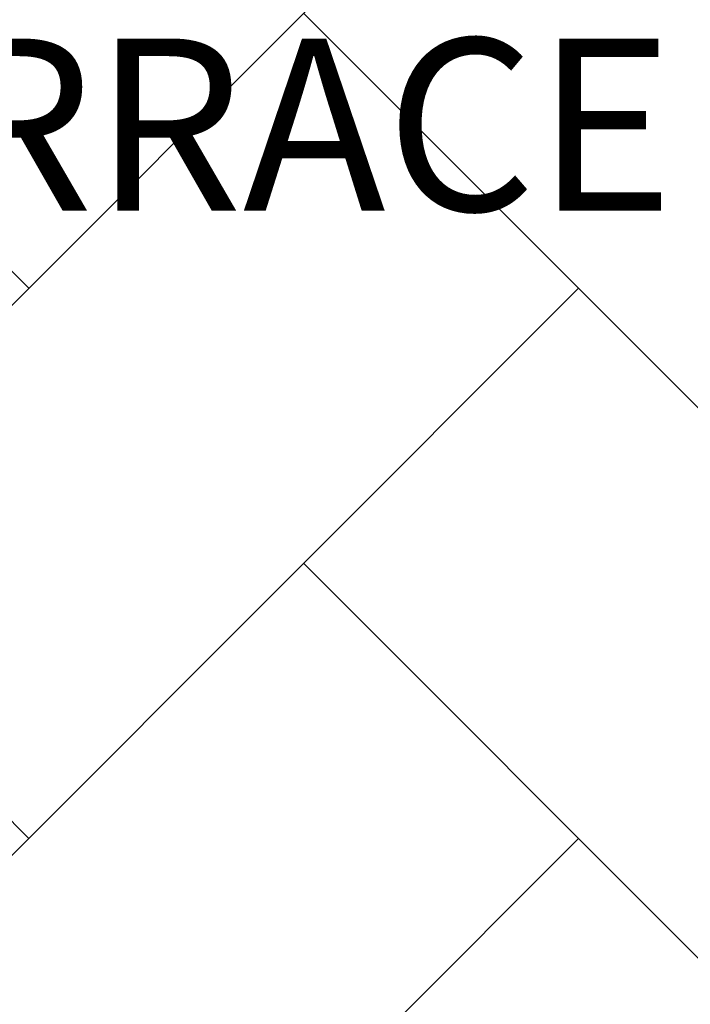
# Model space of a CAD drawing. Units: inches. Extents: x 3590 to 5167, y 65 to 1917.
# Tile 59 of 100: x 5000 to 5035, y 1558 to 1609. Entities that reach past the tile are written whole.
import ezdxf

# ---------------------------------------------------------------- set-up
doc = ezdxf.new("R2010")
doc.units = ezdxf.units.IN
doc.layers.add('A-AREA-IDEN', color=7, linetype='Continuous', lineweight=18)
doc.layers.add('A-FLOR-PATT', color=8, linetype='Continuous', lineweight=13)
doc.styles.get("Standard").update_dxf_attribs({"font": 'arial.ttf'})

msp = doc.modelspace()

# ---------------------------------------------------------------- hatches: boundary and pattern name
at = {"layer": 'A-FLOR-PATT', "transparency": 33554687}
h = msp.add_hatch(dxfattribs=at)
h.set_pattern_fill('AR-HBONE', color=256, scale=0.2)
h.set_pattern_definition([(45, (-588.972, 0), (0, 28.73682), [60.96, -20.32]), (135, (-574.604, 14.368), (3e-15, 28.73682), [60.96, -20.32])])
h.paths.add_polyline_path([(5071.274, 1796.999), (4933.274, 1796.999), (4933.274, 1753.999), (4962.774, 1753.999, -0.414214), (4928.774, 1719.999), (4933.274, 1718.999), (4933.274, 1334.999), (5071.274, 1334.999)])
h.paths.add_polyline_path([(4951.78, 1521.077), (4951.715, 1521.04), (4951.563, 1520.895)], flags=16)
h.paths.add_polyline_path([(4952.267, 1521.376), (4952.198, 1521.371), (4952.198, 1521.356)], flags=0)
h.paths.add_polyline_path([(4967.051, 1529.728), (4965.231, 1528.694), (4963.411, 1527.714), (4961.756, 1526.851), (4963.589, 1527.449), (4964.036, 1527.478), (4962.975, 1527.249), (4961.76, 1526.852), (4959.792, 1525.834), (4958.005, 1524.895), (4956.24, 1523.93), (4954.504, 1522.919), (4954.129, 1522.682), (4953.361, 1521.997), (4953.366, 1521.998), (4953.605, 1522.064), (4955.106, 1522.761), (4956.921, 1523.434), (4958.678, 1523.915), (4960.358, 1524.2), (4961.945, 1524.286), (4964.171, 1524.108), (4965.958, 1523.309), (4963.863, 1522.976), (4965.187, 1522.499), (4963.366, 1522.497), (4961.545, 1522.487), (4959.764, 1522.461), (4958.304, 1522.419), (4957.974, 1522.388), (4956.307, 1522.232), (4954.718, 1522.071), (4953.251, 1521.899), (4953.525, 1521.623), (4954.331, 1521.379), (4956.243, 1521.23), (4958.039, 1520.93), (4959.684, 1520.483), (4961.16, 1519.896), (4963.107, 1518.8), (4964.393, 1517.325), (4962.973, 1517.726), (4964.558, 1516.661), (4965.407, 1515.708), (4963.507, 1516.322), (4961.68, 1517.005), (4959.935, 1517.745), (4958.282, 1518.528), (4956.732, 1519.343), (4955.295, 1520.175), (4954.672, 1520.572), (4954.513, 1520.627), (4955.658, 1519.318), (4956.703, 1517.982), (4957.644, 1516.647), (4958.485, 1515.334), (4959.55, 1513.524), (4960.438, 1511.769), (4958.841, 1513.62), (4957.452, 1515.325), (4955.819, 1517.459), (4956.665, 1515.448), (4957.111, 1513.923), (4957.447, 1511.714), (4957.076, 1509.793), (4956.538, 1511.11), (4955.992, 1512.569), (4955.444, 1514.125), (4954.898, 1515.735), (4954.357, 1517.356), (4953.824, 1518.943), (4953.305, 1520.452), (4953.065, 1521.116), (4952.971, 1521.146), (4952.949, 1521.086), (4952.73, 1520.199), (4953.37, 1518.024), (4953.757, 1516.373), (4954.051, 1514.765), (4954.264, 1513.221), (4954.471, 1511.131), (4954.497, 1510.402), (4954.409, 1511.76), (4954.264, 1513.221), (4954.051, 1514.765), (4953.757, 1516.373), (4953.37, 1518.024), (4952.877, 1519.698), (4952.716, 1520.141), (4952.533, 1519.059), (4952.374, 1517.789), (4952.219, 1516.312), (4952.046, 1514.6), (4951.833, 1512.626), (4951.557, 1510.363), (4951.203, 1512.168), (4950.852, 1514.339), (4950.985, 1516.376), (4951.66, 1518.286), (4952.593, 1520.481), (4952.357, 1521.13), (4951.855, 1520.328), (4950.839, 1518.908), (4949.777, 1517.587), (4948.916, 1516.617), (4948.111, 1515.256), (4947.089, 1513.554), (4945.889, 1511.615), (4946.326, 1513.402), (4946.562, 1514.249), (4945.528, 1513.327), (4944.581, 1512.531), (4946.018, 1514.508), (4947.204, 1516.048), (4947.893, 1517.313), (4949.307, 1518.764), (4950.414, 1519.767), (4950.451, 1519.806), (4952.267, 1521.376), (4951.645, 1521.493), (4950.404, 1521.18), (4948.044, 1520.359), (4946.119, 1519.452), (4944.572, 1518.475), (4943.35, 1517.443), (4941.997, 1515.92), (4941.661, 1515.275), (4942.813, 1516.99), (4944.572, 1518.475), (4946.119, 1519.452), (4948.044, 1520.359), (4950.404, 1521.18), (4951.645, 1521.493), (4949.647, 1521.868), (4948.6, 1521.756), (4947.126, 1521.57), (4945.42, 1521.348), (4943.45, 1521.105), (4941.183, 1520.856), (4942.86, 1521.613), (4943.873, 1522.03), (4942.952, 1521.909), (4941.41, 1521.485), (4939.543, 1520.67), (4938.968, 1520.226), (4940.733, 1521.299), (4942.952, 1521.909), (4943.702, 1522.008), (4945.894, 1522.7), (4947.565, 1522.714), (4948.921, 1522.566), (4951.131, 1522.183), (4950.971, 1522.297), (4948.129, 1523.006), (4946.035, 1523.707), (4944.232, 1524.521), (4942.707, 1525.461), (4941.444, 1526.537), (4940.43, 1527.761), (4939.649, 1529.143), (4941.421, 1528.122), (4943.147, 1527.132), (4944.841, 1526.175), (4946.514, 1525.25), (4948.179, 1524.359), (4948.365, 1524.263), (4946.475, 1526.045), (4945.181, 1527.54), (4944.19, 1529.033), (4943.496, 1530.54), (4943.278, 1531.36), (4942.498, 1531.919), (4943.114, 1531.762), (4942.959, 1533.659), (4944.14, 1531.989), (4944.612, 1531.323), (4946.202, 1530.463), (4947.486, 1529.509), (4948.79, 1528.226), (4950.368, 1526.237), (4949.485, 1528.155), (4948.851, 1530.123), (4948.491, 1532.041), (4948.381, 1533.918), (4948.501, 1535.76), (4948.827, 1537.573), (4949.418, 1535.565), (4949.957, 1533.569), (4950.464, 1531.586), (4950.961, 1529.617), (4951.391, 1527.954), (4951.724, 1530.687), (4952.201, 1532.58), (4952.889, 1534.33), (4953.77, 1535.951), (4954.827, 1537.46), (4954.521, 1535.39), (4954.273, 1533.937), (4955.58, 1535.663), (4956.748, 1536.739), (4956.159, 1534.78), (4955.589, 1532.873), (4955.043, 1531.006), (4954.525, 1529.166), (4954.038, 1527.341), (4953.638, 1525.733), (4953.611, 1525.586), (4953.398, 1524.166), (4953.382, 1524.009), (4954.07, 1525.476), (4954.912, 1527.022), (4956.136, 1528.894), (4957.847, 1530.577), (4959.376, 1531.54), (4958.256, 1530.104), (4957.143, 1528.663), (4956.066, 1527.243), (4955.056, 1525.871), (4954.141, 1524.571), (4953.352, 1523.372), (4953.311, 1523.303), (4953.273, 1522.925), (4953.261, 1522.382), (4954.103, 1523.373), (4954.63, 1524.284), (4955.961, 1526.358), (4957.23, 1528.13), (4958.421, 1529.609), (4960.037, 1531.368), (4961.374, 1532.375), (4962.101, 1532.77), (4961.07, 1531.061), (4959.987, 1529.438), (4958.869, 1527.908), (4958.15, 1527.007), (4959.803, 1528.003), (4961.589, 1528.793), (4963.391, 1529.328), (4965.211, 1529.632)], flags=16)
h.paths.add_polyline_path([(4962.944, 1523.182), (4961.107, 1523.422), (4960.392, 1523.362), (4962.35, 1523.331)], flags=0)
h.paths.add_polyline_path([(5049.541, 1584.551), (5049.476, 1584.515), (5049.325, 1584.37)], flags=16)
h.paths.add_polyline_path([(5050.028, 1584.851), (5049.959, 1584.845), (5049.959, 1584.83)], flags=0)
h.paths.add_polyline_path([(5042.333, 1581.949), (5043.88, 1582.926), (5045.806, 1583.833), (5048.165, 1584.654), (5049.406, 1584.967), (5047.408, 1585.342), (5046.361, 1585.231), (5044.888, 1585.044), (5043.181, 1584.822), (5041.211, 1584.579), (5038.944, 1584.33), (5040.622, 1585.087), (5041.634, 1585.504), (5040.713, 1585.383), (5039.171, 1584.959), (5037.304, 1584.144), (5036.729, 1583.7), (5038.494, 1584.773), (5040.713, 1585.383), (5041.463, 1585.482), (5043.655, 1586.174), (5045.326, 1586.188), (5046.682, 1586.04), (5048.893, 1585.657), (5048.732, 1585.771), (5045.891, 1586.48), (5043.796, 1587.181), (5041.994, 1587.996), (5040.468, 1588.935), (5039.205, 1590.011), (5038.191, 1591.235), (5037.41, 1592.617), (5039.182, 1591.596), (5040.909, 1590.607), (5042.602, 1589.649), (5044.275, 1588.724), (5045.94, 1587.833), (5046.126, 1587.738), (5044.237, 1589.519), (5042.942, 1591.015), (5041.952, 1592.508), (5041.257, 1594.014), (5041.039, 1594.834), (5040.26, 1595.393), (5040.875, 1595.237), (5040.721, 1597.133), (5041.901, 1595.463), (5042.373, 1594.798), (5043.963, 1593.938), (5045.247, 1592.983), (5046.552, 1591.701), (5048.129, 1589.712), (5047.247, 1591.63), (5046.613, 1593.597), (5046.252, 1595.515), (5046.142, 1597.392), (5046.262, 1599.234), (5046.588, 1601.047), (5047.179, 1599.039), (5047.718, 1597.043), (5048.225, 1595.06), (5048.722, 1593.091), (5049.152, 1591.429), (5049.485, 1594.161), (5049.962, 1596.054), (5050.65, 1597.804), (5051.532, 1599.425), (5052.589, 1600.934), (5052.283, 1598.864), (5052.034, 1597.411), (5053.341, 1599.137), (5054.509, 1600.213), (5053.92, 1598.254), (5053.35, 1596.348), (5052.805, 1594.48), (5052.286, 1592.64), (5051.799, 1590.815), (5051.4, 1589.207), (5051.373, 1589.06), (5051.159, 1587.64), (5051.143, 1587.483), (5051.831, 1588.95), (5052.673, 1590.496), (5053.898, 1592.368), (5055.608, 1594.051), (5057.137, 1595.014), (5056.017, 1593.578), (5054.904, 1592.137), (5053.828, 1590.717), (5052.817, 1589.345), (5051.902, 1588.046), (5051.113, 1586.846), (5051.072, 1586.777), (5051.034, 1586.399), (5051.022, 1585.856), (5051.864, 1586.847), (5052.391, 1587.758), (5053.723, 1589.832), (5054.991, 1591.604), (5056.182, 1593.083), (5057.798, 1594.842), (5059.135, 1595.849), (5059.863, 1596.244), (5058.831, 1594.535), (5057.749, 1592.912), (5056.63, 1591.382), (5055.912, 1590.482), (5057.564, 1591.477), (5059.35, 1592.267), (5061.152, 1592.802), (5062.972, 1593.106), (5064.812, 1593.203), (5062.992, 1592.169), (5061.172, 1591.188), (5059.518, 1590.325), (5061.35, 1590.924), (5061.797, 1590.952), (5060.737, 1590.723), (5059.521, 1590.326), (5057.553, 1589.308), (5055.766, 1588.369), (5054.002, 1587.404), (5052.265, 1586.393), (5051.891, 1586.156), (5051.122, 1585.471), (5051.127, 1585.472), (5051.366, 1585.538), (5052.867, 1586.235), (5054.682, 1586.908), (5056.439, 1587.389), (5058.12, 1587.675), (5059.706, 1587.76), (5061.933, 1587.583), (5063.719, 1586.783), (5061.624, 1586.45), (5062.949, 1585.973), (5061.127, 1585.971), (5059.307, 1585.961), (5057.525, 1585.935), (5056.065, 1585.893), (5055.735, 1585.862), (5054.068, 1585.707), (5052.479, 1585.546), (5051.012, 1585.373), (5051.286, 1585.097), (5052.092, 1584.853), (5054.004, 1584.704), (5055.8, 1584.404), (5057.446, 1583.958), (5058.921, 1583.37), (5060.868, 1582.274), (5062.154, 1580.799), (5060.734, 1581.2), (5062.32, 1580.135), (5063.168, 1579.182), (5061.269, 1579.796), (5059.441, 1580.479), (5057.696, 1581.219), (5056.043, 1582.003), (5054.493, 1582.817), (5053.057, 1583.649), (5052.433, 1584.047), (5052.274, 1584.101), (5053.42, 1582.793), (5054.464, 1581.457), (5055.405, 1580.121), (5056.247, 1578.809), (5057.311, 1576.998), (5058.199, 1575.244), (5056.602, 1577.094), (5055.213, 1578.799), (5053.58, 1580.933), (5054.427, 1578.922), (5054.872, 1577.397), (5055.208, 1575.189), (5054.838, 1573.267), (5054.299, 1574.584), (5053.754, 1576.043), (5053.206, 1577.599), (5052.659, 1579.209), (5052.118, 1580.83), (5051.585, 1582.417), (5051.066, 1583.927), (5050.826, 1584.59), (5050.733, 1584.62), (5050.711, 1584.561), (5050.491, 1583.673), (5051.131, 1581.498), (5051.518, 1579.847), (5051.813, 1578.24), (5052.026, 1576.695), (5052.233, 1574.605), (5052.258, 1573.876), (5052.17, 1575.234), (5052.026, 1576.695), (5051.813, 1578.24), (5051.518, 1579.847), (5051.131, 1581.498), (5050.638, 1583.172), (5050.477, 1583.615), (5050.294, 1582.533), (5050.136, 1581.263), (5049.981, 1579.786), (5049.807, 1578.074), (5049.594, 1576.1), (5049.318, 1573.837), (5048.965, 1575.642), (5048.613, 1577.813), (5048.747, 1579.85), (5049.421, 1581.76), (5050.354, 1583.955), (5050.118, 1584.604), (5049.616, 1583.802), (5048.6, 1582.382), (5047.538, 1581.061), (5046.677, 1580.091), (5045.872, 1578.73), (5044.85, 1577.028), (5043.651, 1575.089), (5044.087, 1576.877), (5044.324, 1577.723), (5043.289, 1576.801), (5042.342, 1576.005), (5043.779, 1577.982), (5044.966, 1579.522), (5045.655, 1580.787), (5047.068, 1582.239), (5048.175, 1583.241), (5048.213, 1583.28), (5050.028, 1584.851), (5049.406, 1584.967), (5048.165, 1584.654), (5045.806, 1583.833), (5043.88, 1582.926), (5042.333, 1581.949), (5041.111, 1580.917), (5039.758, 1579.394), (5039.423, 1578.749), (5040.575, 1580.464)], flags=16)
h.paths.add_polyline_path([(4954.799, 1533.12), (4954.262, 1532.079), (4953.831, 1530.935), (4953.505, 1529.636), (4953.283, 1528.133), (4953.167, 1526.376), (4953.156, 1524.315), (4953.277, 1521.236), (4952.802, 1521.842), (4951.557, 1521.998), (4950.976, 1521.961), (4952.661, 1521.941), (4952.802, 1521.842), (4953.152, 1523.593), (4953.167, 1526.376), (4953.283, 1528.133), (4953.609, 1530.346), (4954.456, 1532.592)], flags=0)
h.paths.add_polyline_path([(5050.563, 1585.316), (5049.318, 1585.472), (5048.737, 1585.435), (5050.422, 1585.415), (5050.563, 1585.316), (5050.914, 1587.067), (5050.928, 1589.851), (5051.045, 1591.607), (5051.371, 1593.82), (5052.217, 1596.066), (5052.56, 1596.594), (5052.024, 1595.554), (5051.592, 1594.409), (5051.266, 1593.11), (5051.045, 1591.607), (5050.928, 1589.851), (5050.918, 1587.789), (5051.038, 1584.71)], flags=0)
h.paths.add_polyline_path([(5058.153, 1586.836), (5060.111, 1586.805), (5060.705, 1586.656), (5058.868, 1586.896)], flags=0)
h.paths.add_polyline_path([(5049.541, 1430.936), (5049.476, 1430.9), (5049.325, 1430.755)], flags=16)
h.paths.add_polyline_path([(5050.028, 1431.236), (5049.959, 1431.231), (5049.959, 1431.215)], flags=0)
h.paths.add_polyline_path([(5046.588, 1447.432), (5047.179, 1445.425), (5047.718, 1443.429), (5048.225, 1441.446), (5048.722, 1439.476), (5049.152, 1437.814), (5049.485, 1440.546), (5049.962, 1442.439), (5050.65, 1444.189), (5051.532, 1445.811), (5052.589, 1447.319), (5052.283, 1445.249), (5052.034, 1443.796), (5053.341, 1445.522), (5054.509, 1446.598), (5053.92, 1444.64), (5053.35, 1442.733), (5052.805, 1440.865), (5052.286, 1439.025), (5051.799, 1437.201), (5051.4, 1435.592), (5051.373, 1435.445), (5051.159, 1434.025), (5051.143, 1433.868), (5051.831, 1435.335), (5052.673, 1436.881), (5053.898, 1438.753), (5055.608, 1440.436), (5057.137, 1441.4), (5056.017, 1439.963), (5054.904, 1438.522), (5053.828, 1437.102), (5052.817, 1435.73), (5051.902, 1434.431), (5051.113, 1433.231), (5051.072, 1433.162), (5051.034, 1432.784), (5051.022, 1432.242), (5051.864, 1433.232), (5052.391, 1434.143), (5053.723, 1436.217), (5054.991, 1437.989), (5056.182, 1439.468), (5057.798, 1441.227), (5059.135, 1442.235), (5059.863, 1442.629), (5058.831, 1440.921), (5057.749, 1439.298), (5056.63, 1437.767), (5055.912, 1436.867), (5057.564, 1437.863), (5059.35, 1438.652), (5061.152, 1439.187), (5062.972, 1439.491), (5064.812, 1439.588), (5062.992, 1438.554), (5061.172, 1437.573), (5059.518, 1436.71), (5061.35, 1437.309), (5061.797, 1437.337), (5060.737, 1437.108), (5059.521, 1436.711), (5057.553, 1435.693), (5055.766, 1434.754), (5054.002, 1433.789), (5052.265, 1432.778), (5051.891, 1432.541), (5051.122, 1431.856), (5051.127, 1431.857), (5051.366, 1431.923), (5052.867, 1432.62), (5054.682, 1433.293), (5056.439, 1433.775), (5058.12, 1434.06), (5059.706, 1434.145), (5061.933, 1433.968), (5063.719, 1433.168), (5061.624, 1432.835), (5062.949, 1432.358), (5061.127, 1432.357), (5059.307, 1432.346), (5057.525, 1432.32), (5056.065, 1432.278), (5055.735, 1432.248), (5054.068, 1432.092), (5052.479, 1431.931), (5051.012, 1431.759), (5051.286, 1431.482), (5052.092, 1431.238), (5054.004, 1431.089), (5055.8, 1430.789), (5057.446, 1430.343), (5058.921, 1429.755), (5060.868, 1428.66), (5062.154, 1427.185), (5060.734, 1427.585), (5062.32, 1426.52), (5063.168, 1425.567), (5061.269, 1426.181), (5059.441, 1426.865), (5057.696, 1427.604), (5056.043, 1428.388), (5054.493, 1429.202), (5053.057, 1430.034), (5052.433, 1430.432), (5052.274, 1430.487), (5053.42, 1429.178), (5054.464, 1427.842), (5055.405, 1426.506), (5056.247, 1425.194), (5057.311, 1423.383), (5058.199, 1421.629), (5056.602, 1423.479), (5055.213, 1425.184), (5053.58, 1427.318), (5054.427, 1425.307), (5054.872, 1423.782), (5055.208, 1421.574), (5054.838, 1419.652), (5054.299, 1420.97), (5053.754, 1422.428), (5053.206, 1423.984), (5052.659, 1425.595), (5052.118, 1427.215), (5051.585, 1428.802), (5051.066, 1430.312), (5050.826, 1430.975), (5050.733, 1431.005), (5050.711, 1430.946), (5050.491, 1430.058), (5051.131, 1427.883), (5051.518, 1426.232), (5051.813, 1424.625), (5052.026, 1423.081), (5052.233, 1420.991), (5052.258, 1420.261), (5052.17, 1421.619), (5052.026, 1423.081), (5051.813, 1424.625), (5051.518, 1426.232), (5051.131, 1427.883), (5050.638, 1429.558), (5050.477, 1430.001), (5050.294, 1428.918), (5050.136, 1427.648), (5049.981, 1426.171), (5049.807, 1424.459), (5049.594, 1422.485), (5049.318, 1420.222), (5048.965, 1422.028), (5048.613, 1424.199), (5048.747, 1426.235), (5049.421, 1428.146), (5050.354, 1430.34), (5050.118, 1430.989), (5049.616, 1430.187), (5048.6, 1428.768), (5047.538, 1427.446), (5046.677, 1426.477), (5045.872, 1425.116), (5044.85, 1423.413), (5043.651, 1421.474), (5044.087, 1423.262), (5044.324, 1424.109), (5043.289, 1423.186), (5042.342, 1422.391), (5043.779, 1424.368), (5044.966, 1425.907), (5045.655, 1427.173), (5047.068, 1428.624), (5048.175, 1429.627), (5048.213, 1429.666), (5050.028, 1431.236), (5049.406, 1431.353), (5048.165, 1431.039), (5045.806, 1430.218), (5043.88, 1429.311), (5042.333, 1428.334), (5041.111, 1427.302), (5039.758, 1425.779), (5039.423, 1425.134), (5040.575, 1426.849), (5042.333, 1428.334), (5043.88, 1429.311), (5045.806, 1430.218), (5048.165, 1431.039), (5049.406, 1431.353), (5047.408, 1431.727), (5046.361, 1431.616), (5044.888, 1431.429), (5043.181, 1431.207), (5041.211, 1430.964), (5038.944, 1430.715), (5040.622, 1431.472), (5041.634, 1431.89), (5040.713, 1431.769), (5039.171, 1431.345), (5037.304, 1430.53), (5036.729, 1430.085), (5038.494, 1431.158), (5040.713, 1431.769), (5041.463, 1431.867), (5043.655, 1432.559), (5045.326, 1432.573), (5046.682, 1432.425), (5048.893, 1432.042), (5048.732, 1432.156), (5045.891, 1432.865), (5043.796, 1433.566), (5041.994, 1434.381), (5040.468, 1435.321), (5039.205, 1436.396), (5038.191, 1437.62), (5037.41, 1439.002), (5039.182, 1437.982), (5040.909, 1436.992), (5042.602, 1436.034), (5044.275, 1435.109), (5045.94, 1434.218), (5046.126, 1434.123), (5044.237, 1435.904), (5042.942, 1437.4), (5041.952, 1438.893), (5041.257, 1440.399), (5041.039, 1441.219), (5040.26, 1441.778), (5040.875, 1441.622), (5040.721, 1443.518), (5041.901, 1441.848), (5042.373, 1441.183), (5043.963, 1440.323), (5045.247, 1439.369), (5046.552, 1438.086), (5048.129, 1436.097), (5047.247, 1438.015), (5046.613, 1439.982), (5046.252, 1441.901), (5046.142, 1443.778), (5046.262, 1445.619)], flags=16)
h.paths.add_polyline_path([(5052.382, 1444.255), (5051.623, 1442.78), (5052.024, 1441.939), (5052.56, 1442.98)], flags=0)
h.paths.add_polyline_path([(5050.563, 1431.701), (5049.318, 1431.857), (5048.737, 1431.821), (5050.422, 1431.8)], flags=0)
h.paths.add_polyline_path([(5058.153, 1433.221), (5060.111, 1433.19), (5060.705, 1433.041), (5058.868, 1433.281)], flags=0)
h.paths.add_polyline_path([(5049.541, 1352.285), (5049.476, 1352.249), (5049.325, 1352.104)], flags=16)
h.paths.add_polyline_path([(5050.028, 1352.585), (5049.959, 1352.58), (5049.959, 1352.564)], flags=0)
h.paths.add_polyline_path([(5046.588, 1368.781), (5047.179, 1366.774), (5047.718, 1364.778), (5048.225, 1362.795), (5048.722, 1360.825), (5049.152, 1359.163), (5049.485, 1361.896), (5049.962, 1363.789), (5050.65, 1365.538), (5051.532, 1367.16), (5052.589, 1368.669), (5052.283, 1366.598), (5052.034, 1365.145), (5053.341, 1366.871), (5054.509, 1367.947), (5053.92, 1365.989), (5053.35, 1364.082), (5052.805, 1362.214), (5052.286, 1360.374), (5051.799, 1358.55), (5051.4, 1356.942), (5051.373, 1356.794), (5051.159, 1355.374), (5051.143, 1355.218), (5051.831, 1356.684), (5052.673, 1358.23), (5053.898, 1360.102), (5055.608, 1361.786), (5057.137, 1362.749), (5056.017, 1361.313), (5054.904, 1359.872), (5053.828, 1358.452), (5052.817, 1357.079), (5051.902, 1355.78), (5051.113, 1354.581), (5051.072, 1354.512), (5051.034, 1354.133), (5051.022, 1353.591), (5051.864, 1354.581), (5052.391, 1355.492), (5053.723, 1357.566), (5054.991, 1359.338), (5056.182, 1360.817), (5057.798, 1362.577), (5059.135, 1363.584), (5059.863, 1363.979), (5058.831, 1362.27), (5057.749, 1360.647), (5056.63, 1359.117), (5055.912, 1358.216), (5057.564, 1359.212), (5059.35, 1360.001), (5061.152, 1360.536), (5062.972, 1360.841), (5064.812, 1360.937), (5062.992, 1359.903), (5061.172, 1358.923), (5059.518, 1358.059), (5061.35, 1358.658), (5061.797, 1358.687), (5060.737, 1358.458), (5059.521, 1358.061), (5057.553, 1357.043), (5055.766, 1356.103), (5054.002, 1355.138), (5052.265, 1354.127), (5051.891, 1353.89), (5051.122, 1353.206), (5051.127, 1353.206), (5051.366, 1353.272), (5052.867, 1353.969), (5054.682, 1354.643), (5056.439, 1355.124), (5058.12, 1355.409), (5059.706, 1355.495), (5061.933, 1355.317), (5063.719, 1354.518), (5061.624, 1354.184), (5062.949, 1353.708), (5061.127, 1353.706), (5059.307, 1353.695), (5057.525, 1353.669), (5056.065, 1353.627), (5055.735, 1353.597), (5054.068, 1353.441), (5052.479, 1353.28), (5051.012, 1353.108), (5051.286, 1352.831), (5052.092, 1352.587), (5054.004, 1352.439), (5055.8, 1352.138), (5057.446, 1351.692), (5058.921, 1351.104), (5060.868, 1350.009), (5062.154, 1348.534), (5060.734, 1348.935), (5062.32, 1347.869), (5063.168, 1346.916), (5061.269, 1347.53), (5059.441, 1348.214), (5057.696, 1348.954), (5056.043, 1349.737), (5054.493, 1350.551), (5053.057, 1351.383), (5052.433, 1351.781), (5052.274, 1351.836), (5053.42, 1350.527), (5054.464, 1349.191), (5055.405, 1347.855), (5056.247, 1346.543), (5057.311, 1344.733), (5058.199, 1342.978), (5056.602, 1344.828), (5055.213, 1346.534), (5053.58, 1348.667), (5054.427, 1346.656), (5054.872, 1345.132), (5055.208, 1342.923), (5054.838, 1341.002), (5054.299, 1342.319), (5053.754, 1343.778), (5053.206, 1345.334), (5052.659, 1346.944), (5052.118, 1348.564), (5051.585, 1350.151), (5051.066, 1351.661), (5050.826, 1352.324), (5050.733, 1352.355), (5050.711, 1352.295), (5050.491, 1351.408), (5051.131, 1349.232), (5051.518, 1347.581), (5051.813, 1345.974), (5052.026, 1344.43), (5052.233, 1342.34), (5052.258, 1341.61), (5052.17, 1342.969), (5052.026, 1344.43), (5051.813, 1345.974), (5051.518, 1347.581), (5051.131, 1349.232), (5050.638, 1350.907), (5050.477, 1351.35), (5050.294, 1350.267), (5050.136, 1348.997), (5049.981, 1347.52), (5049.807, 1345.809), (5049.594, 1343.835), (5049.318, 1341.571), (5048.965, 1343.377), (5048.613, 1345.548), (5048.747, 1347.585), (5049.421, 1349.495), (5050.354, 1351.689), (5050.118, 1352.339), (5049.616, 1351.536), (5048.6, 1350.117), (5047.538, 1348.795), (5046.677, 1347.826), (5045.872, 1346.465), (5044.85, 1344.763), (5043.651, 1342.824), (5044.087, 1344.611), (5044.324, 1345.458), (5043.289, 1344.535), (5042.342, 1343.74), (5043.779, 1345.717), (5044.966, 1347.256), (5045.655, 1348.522), (5047.068, 1349.973), (5048.175, 1350.976), (5048.213, 1351.015), (5050.028, 1352.585), (5049.406, 1352.702), (5048.165, 1352.388), (5045.806, 1351.567), (5043.88, 1350.661), (5042.333, 1349.683), (5041.111, 1348.651), (5039.758, 1347.128), (5039.423, 1346.483), (5040.575, 1348.198), (5042.333, 1349.683), (5043.88, 1350.661), (5045.806, 1351.567), (5048.165, 1352.388), (5049.406, 1352.702), (5047.408, 1353.076), (5046.361, 1352.965), (5044.888, 1352.779), (5043.181, 1352.556), (5041.211, 1352.313), (5038.944, 1352.065), (5040.622, 1352.821), (5041.634, 1353.239), (5040.713, 1353.118), (5039.171, 1352.694), (5037.304, 1351.879), (5036.729, 1351.434), (5038.494, 1352.508), (5040.713, 1353.118), (5041.463, 1353.216), (5043.655, 1353.909), (5045.326, 1353.923), (5046.682, 1353.774), (5048.893, 1353.391), (5048.732, 1353.506), (5045.891, 1354.214), (5043.796, 1354.915), (5041.994, 1355.73), (5040.468, 1356.67), (5039.205, 1357.746), (5038.191, 1358.969), (5037.41, 1360.352), (5039.182, 1359.331), (5040.909, 1358.341), (5042.602, 1357.383), (5044.275, 1356.458), (5045.94, 1355.567), (5046.126, 1355.472), (5044.237, 1357.253), (5042.942, 1358.749), (5041.952, 1360.242), (5041.257, 1361.748), (5041.039, 1362.568), (5040.26, 1363.128), (5040.875, 1362.971), (5040.721, 1364.867), (5041.901, 1363.197), (5042.373, 1362.532), (5043.963, 1361.672), (5045.247, 1360.718), (5046.552, 1359.435), (5048.129, 1357.446), (5047.247, 1359.364), (5046.613, 1361.331), (5046.252, 1363.25), (5046.142, 1365.127), (5046.262, 1366.969)], flags=16)
h.paths.add_polyline_path([(5052.382, 1365.604), (5051.623, 1364.129), (5052.024, 1363.288), (5052.56, 1364.329)], flags=0)
h.paths.add_polyline_path([(4951.78, 1698.041), (4951.715, 1698.005), (4951.563, 1697.859)], flags=16)
h.paths.add_polyline_path([(4952.267, 1698.341), (4952.198, 1698.335), (4952.198, 1698.32)], flags=0)
h.paths.add_polyline_path([(4957.076, 1686.757), (4956.538, 1688.074), (4955.992, 1689.533), (4955.444, 1691.089), (4954.898, 1692.699), (4954.357, 1694.32), (4953.824, 1695.907), (4953.305, 1697.417), (4953.065, 1698.08), (4952.971, 1698.11), (4952.949, 1698.051), (4952.73, 1697.163), (4953.37, 1694.988), (4953.757, 1693.337), (4954.051, 1691.729), (4954.264, 1690.185), (4954.471, 1688.095), (4954.497, 1687.366), (4954.409, 1688.724), (4954.264, 1690.185), (4954.051, 1691.729), (4953.757, 1693.337), (4953.37, 1694.988), (4952.877, 1696.662), (4952.716, 1697.105), (4952.533, 1696.023), (4952.374, 1694.753), (4952.219, 1693.276), (4952.046, 1691.564), (4951.833, 1689.59), (4951.557, 1687.327), (4951.203, 1689.132), (4950.852, 1691.303), (4950.985, 1693.34), (4951.66, 1695.25), (4952.593, 1697.445), (4952.357, 1698.094), (4951.855, 1697.292), (4950.839, 1695.872), (4949.777, 1694.551), (4948.916, 1693.581), (4948.111, 1692.22), (4947.089, 1690.518), (4945.889, 1688.579), (4946.326, 1690.366), (4946.562, 1691.213), (4945.528, 1690.291), (4944.581, 1689.495), (4946.018, 1691.472), (4947.204, 1693.012), (4947.893, 1694.277), (4949.307, 1695.729), (4950.414, 1696.731), (4950.451, 1696.77), (4952.267, 1698.341), (4951.645, 1698.457), (4950.404, 1698.144), (4948.044, 1697.323), (4946.119, 1696.416), (4944.572, 1695.439), (4943.35, 1694.407), (4941.997, 1692.884), (4941.661, 1692.239), (4942.813, 1693.954), (4944.572, 1695.439), (4946.119, 1696.416), (4948.044, 1697.323), (4950.404, 1698.144), (4951.645, 1698.457), (4949.647, 1698.832), (4948.6, 1698.72), (4947.126, 1698.534), (4945.42, 1698.312), (4943.45, 1698.069), (4941.183, 1697.82), (4942.86, 1698.577), (4943.873, 1698.994), (4942.952, 1698.873), (4941.41, 1698.449), (4939.543, 1697.634), (4938.968, 1697.19), (4940.733, 1698.263), (4942.952, 1698.873), (4943.702, 1698.972), (4945.894, 1699.664), (4947.565, 1699.678), (4948.921, 1699.53), (4951.131, 1699.147), (4950.971, 1699.261), (4948.129, 1699.97), (4946.035, 1700.671), (4944.232, 1701.486), (4942.707, 1702.425), (4941.444, 1703.501), (4940.43, 1704.725), (4939.649, 1706.107), (4941.421, 1705.086), (4943.147, 1704.097), (4944.841, 1703.139), (4946.514, 1702.214), (4948.179, 1701.323), (4948.365, 1701.227), (4946.475, 1703.009), (4945.181, 1704.505), (4944.19, 1705.997), (4943.496, 1707.504), (4943.278, 1708.324), (4942.498, 1708.883), (4943.114, 1708.727), (4942.959, 1710.623), (4944.14, 1708.953), (4944.612, 1708.287), (4946.202, 1707.428), (4947.486, 1706.473), (4948.79, 1705.191), (4950.368, 1703.202), (4949.485, 1705.12), (4948.851, 1707.087), (4948.491, 1709.005), (4948.381, 1710.882), (4948.501, 1712.724), (4948.827, 1714.537), (4949.418, 1712.529), (4949.957, 1710.533), (4950.464, 1708.55), (4950.961, 1706.581), (4951.391, 1704.919), (4951.724, 1707.651), (4952.201, 1709.544), (4952.889, 1711.294), (4953.77, 1712.915), (4954.827, 1714.424), (4954.521, 1712.354), (4954.273, 1710.901), (4955.58, 1712.627), (4956.748, 1713.703), (4956.159, 1711.744), (4955.589, 1709.837), (4955.043, 1707.97), (4954.525, 1706.13), (4954.038, 1704.305), (4953.638, 1702.697), (4953.611, 1702.55), (4953.398, 1701.13), (4953.382, 1700.973), (4954.07, 1702.44), (4954.912, 1703.986), (4956.136, 1705.858), (4957.847, 1707.541), (4959.376, 1708.504), (4958.256, 1707.068), (4957.143, 1705.627), (4956.066, 1704.207), (4955.056, 1702.835), (4954.141, 1701.536), (4953.352, 1700.336), (4953.311, 1700.267), (4953.273, 1699.889), (4953.261, 1699.346), (4954.103, 1700.337), (4954.63, 1701.248), (4955.961, 1703.322), (4957.23, 1705.094), (4958.421, 1706.573), (4960.037, 1708.332), (4961.374, 1709.339), (4962.101, 1709.734), (4961.07, 1708.025), (4959.987, 1706.402), (4958.869, 1704.872), (4958.15, 1703.972), (4959.803, 1704.967), (4961.589, 1705.757), (4963.391, 1706.292), (4965.211, 1706.596), (4967.051, 1706.692), (4965.231, 1705.659), (4963.411, 1704.678), (4961.756, 1703.815), (4963.589, 1704.413), (4964.036, 1704.442), (4962.975, 1704.213), (4961.76, 1703.816), (4959.792, 1702.798), (4958.005, 1701.859), (4956.24, 1700.894), (4954.504, 1699.883), (4954.129, 1699.646), (4953.361, 1698.961), (4953.366, 1698.962), (4953.605, 1699.028), (4955.106, 1699.725), (4956.921, 1700.398), (4958.678, 1700.879), (4960.358, 1701.164), (4961.945, 1701.25), (4964.171, 1701.073), (4965.958, 1700.273), (4963.863, 1699.94), (4965.187, 1699.463), (4963.366, 1699.461), (4961.545, 1699.451), (4959.764, 1699.425), (4958.304, 1699.383), (4957.974, 1699.352), (4956.307, 1699.197), (4954.718, 1699.036), (4953.251, 1698.863), (4953.525, 1698.587), (4954.331, 1698.343), (4956.243, 1698.194), (4958.039, 1697.894), (4959.684, 1697.447), (4961.16, 1696.86), (4963.107, 1695.764), (4964.393, 1694.289), (4962.973, 1694.69), (4964.558, 1693.625), (4965.407, 1692.672), (4963.507, 1693.286), (4961.68, 1693.969), (4959.935, 1694.709), (4958.282, 1695.492), (4956.732, 1696.307), (4955.295, 1697.139), (4954.672, 1697.536), (4954.513, 1697.591), (4955.658, 1696.282), (4956.703, 1694.946), (4957.644, 1693.611), (4958.485, 1692.298), (4959.55, 1690.488), (4960.438, 1688.733), (4958.841, 1690.584), (4957.452, 1692.289), (4955.819, 1694.423), (4956.665, 1692.412), (4957.111, 1690.887), (4957.447, 1688.678)], flags=16)
h.paths.add_polyline_path([(5050.563, 1353.05), (5049.318, 1353.207), (5048.737, 1353.17), (5050.422, 1353.15)], flags=0)
h.paths.add_polyline_path([(4951.78, 1351.486), (4951.715, 1351.45), (4951.563, 1351.305)], flags=16)
h.paths.add_polyline_path([(4952.267, 1351.786), (4952.198, 1351.78), (4952.198, 1351.765)], flags=0)
h.paths.add_polyline_path([(4954.827, 1367.869), (4954.521, 1365.799), (4954.273, 1364.346), (4955.58, 1366.072), (4956.748, 1367.148), (4956.159, 1365.19), (4955.589, 1363.283), (4955.043, 1361.415), (4954.525, 1359.575), (4954.038, 1357.751), (4953.638, 1356.142), (4953.611, 1355.995), (4953.398, 1354.575), (4953.382, 1354.418), (4954.07, 1355.885), (4954.912, 1357.431), (4956.136, 1359.303), (4957.847, 1360.986), (4959.376, 1361.95), (4958.256, 1360.513), (4957.143, 1359.072), (4956.066, 1357.652), (4955.056, 1356.28), (4954.141, 1354.981), (4953.352, 1353.781), (4953.311, 1353.712), (4953.273, 1353.334), (4953.261, 1352.792), (4954.103, 1353.782), (4954.63, 1354.693), (4955.961, 1356.767), (4957.23, 1358.539), (4958.421, 1360.018), (4960.037, 1361.777), (4961.374, 1362.785), (4962.101, 1363.179), (4961.07, 1361.471), (4959.987, 1359.848), (4958.869, 1358.317), (4958.15, 1357.417), (4959.803, 1358.413), (4961.589, 1359.202), (4963.391, 1359.737), (4965.211, 1360.041), (4967.051, 1360.138), (4965.231, 1359.104), (4963.411, 1358.123), (4961.756, 1357.26), (4963.589, 1357.859), (4964.036, 1357.887), (4962.975, 1357.658), (4961.76, 1357.261), (4959.792, 1356.243), (4958.005, 1355.304), (4956.24, 1354.339), (4954.504, 1353.328), (4954.129, 1353.091), (4953.361, 1352.406), (4953.366, 1352.407), (4953.605, 1352.473), (4955.106, 1353.17), (4956.921, 1353.843), (4958.678, 1354.325), (4960.358, 1354.61), (4961.945, 1354.695), (4964.171, 1354.518), (4965.958, 1353.718), (4963.863, 1353.385), (4965.187, 1352.908), (4963.366, 1352.907), (4961.545, 1352.896), (4959.764, 1352.87), (4958.304, 1352.828), (4957.974, 1352.798), (4956.307, 1352.642), (4954.718, 1352.481), (4953.251, 1352.309), (4953.525, 1352.032), (4954.331, 1351.788), (4956.243, 1351.639), (4958.039, 1351.339), (4959.684, 1350.893), (4961.16, 1350.305), (4963.107, 1349.21), (4964.393, 1347.735), (4962.973, 1348.135), (4964.558, 1347.07), (4965.407, 1346.117), (4963.507, 1346.731), (4961.68, 1347.414), (4959.935, 1348.154), (4958.282, 1348.938), (4956.732, 1349.752), (4955.295, 1350.584), (4954.672, 1350.982), (4954.513, 1351.036), (4955.658, 1349.728), (4956.703, 1348.392), (4957.644, 1347.056), (4958.485, 1345.744), (4959.55, 1343.933), (4960.438, 1342.179), (4958.841, 1344.029), (4957.452, 1345.734), (4955.819, 1347.868), (4956.665, 1345.857), (4957.111, 1344.332), (4957.447, 1342.124), (4957.076, 1340.202), (4956.538, 1341.52), (4955.992, 1342.978), (4955.444, 1344.534), (4954.898, 1346.145), (4954.357, 1347.765), (4953.824, 1349.352), (4953.305, 1350.862), (4953.065, 1351.525), (4952.971, 1351.555), (4952.949, 1351.496), (4952.73, 1350.608), (4953.37, 1348.433), (4953.757, 1346.782), (4954.051, 1345.175), (4954.264, 1343.631), (4954.471, 1341.541), (4954.497, 1340.811), (4954.409, 1342.169), (4954.264, 1343.631), (4954.051, 1345.175), (4953.757, 1346.782), (4953.37, 1348.433), (4952.877, 1350.108), (4952.716, 1350.551), (4952.533, 1349.468), (4952.374, 1348.198), (4952.219, 1346.721), (4952.046, 1345.009), (4951.833, 1343.035), (4951.557, 1340.772), (4951.203, 1342.578), (4950.852, 1344.749), (4950.985, 1346.785), (4951.66, 1348.696), (4952.593, 1350.89), (4952.357, 1351.539), (4951.855, 1350.737), (4950.839, 1349.318), (4949.777, 1347.996), (4948.916, 1347.027), (4948.111, 1345.665), (4947.089, 1343.963), (4945.889, 1342.024), (4946.326, 1343.812), (4946.562, 1344.659), (4945.528, 1343.736), (4944.581, 1342.941), (4946.018, 1344.918), (4947.204, 1346.457), (4947.893, 1347.723), (4949.307, 1349.174), (4950.414, 1350.177), (4950.451, 1350.216), (4952.267, 1351.786), (4951.645, 1351.903), (4950.404, 1351.589), (4948.044, 1350.768), (4946.119, 1349.861), (4944.572, 1348.884), (4943.35, 1347.852), (4941.997, 1346.329), (4941.661, 1345.684), (4942.813, 1347.399), (4944.572, 1348.884), (4946.119, 1349.861), (4948.044, 1350.768), (4950.404, 1351.589), (4951.645, 1351.903), (4949.647, 1352.277), (4948.6, 1352.166), (4947.126, 1351.979), (4945.42, 1351.757), (4943.45, 1351.514), (4941.183, 1351.265), (4942.86, 1352.022), (4943.873, 1352.44), (4942.952, 1352.319), (4941.41, 1351.895), (4939.543, 1351.08), (4938.968, 1350.635), (4940.733, 1351.708), (4942.952, 1352.319), (4943.702, 1352.417), (4945.894, 1353.109), (4947.565, 1353.123), (4948.921, 1352.975), (4951.131, 1352.592), (4950.971, 1352.706), (4948.129, 1353.415), (4946.035, 1354.116), (4944.232, 1354.931), (4942.707, 1355.871), (4941.444, 1356.946), (4940.43, 1358.17), (4939.649, 1359.552), (4941.421, 1358.532), (4943.147, 1357.542), (4944.841, 1356.584), (4946.514, 1355.659), (4948.179, 1354.768), (4948.365, 1354.673), (4946.475, 1356.454), (4945.181, 1357.95), (4944.19, 1359.443), (4943.496, 1360.949), (4943.278, 1361.769), (4942.498, 1362.328), (4943.114, 1362.172), (4942.959, 1364.068), (4944.14, 1362.398), (4944.612, 1361.733), (4946.202, 1360.873), (4947.486, 1359.919), (4948.79, 1358.636), (4950.368, 1356.647), (4949.485, 1358.565), (4948.851, 1360.532), (4948.491, 1362.451), (4948.381, 1364.328), (4948.501, 1366.169), (4948.827, 1367.982), (4949.418, 1365.975), (4949.957, 1363.979), (4950.464, 1361.995), (4950.961, 1360.026), (4951.391, 1358.364), (4951.724, 1361.096), (4952.201, 1362.989), (4952.889, 1364.739), (4953.77, 1366.361)], flags=16)
h.paths.add_polyline_path([(4954.799, 1363.53), (4954.262, 1362.489), (4953.831, 1361.344), (4953.505, 1360.045), (4953.283, 1358.543), (4953.167, 1356.786), (4953.156, 1354.724), (4953.277, 1351.646), (4952.802, 1352.251), (4951.557, 1352.407), (4950.976, 1352.371), (4952.661, 1352.35), (4952.802, 1352.251), (4953.152, 1354.002), (4953.167, 1356.786), (4953.283, 1358.543), (4953.609, 1360.755), (4954.456, 1363.001)], flags=0)
h.paths.add_polyline_path([(4952.802, 1698.806), (4951.557, 1698.962), (4950.976, 1698.925), (4952.661, 1698.905), (4952.802, 1698.806), (4953.152, 1700.557), (4953.167, 1703.34), (4953.283, 1705.097), (4953.609, 1707.31), (4954.456, 1709.556), (4954.799, 1710.084), (4954.262, 1709.043), (4953.831, 1707.899), (4953.505, 1706.6), (4953.283, 1705.097), (4953.167, 1703.34), (4953.156, 1701.279), (4953.277, 1698.2)], flags=0)
h.paths.add_polyline_path([(4962.944, 1700.146), (4961.107, 1700.386), (4960.392, 1700.326), (4962.35, 1700.295)], flags=0)
h.paths.add_polyline_path([(5058.153, 1354.57), (5060.111, 1354.539), (5060.705, 1354.391), (5058.868, 1354.631)], flags=0)
h.paths.add_polyline_path([(4962.944, 1353.591), (4961.107, 1353.831), (4960.392, 1353.771), (4962.35, 1353.74)], flags=0)
h.paths.add_polyline_path([(5049.541, 1778.72), (5049.476, 1778.684), (5049.325, 1778.539)], flags=16)
h.paths.add_polyline_path([(5050.028, 1779.02), (5049.959, 1779.014), (5049.959, 1778.999)], flags=0)
h.paths.add_polyline_path([(5052.258, 1768.045), (5052.17, 1769.403), (5052.026, 1770.864), (5051.813, 1772.409), (5051.518, 1774.016), (5051.131, 1775.667), (5050.638, 1777.341), (5050.477, 1777.784), (5050.294, 1776.702), (5050.136, 1775.432), (5049.981, 1773.955), (5049.807, 1772.243), (5049.594, 1770.269), (5049.318, 1768.006), (5048.965, 1769.811), (5048.613, 1771.982), (5048.747, 1774.019), (5049.421, 1775.929), (5050.354, 1778.124), (5050.118, 1778.773), (5049.616, 1777.971), (5048.6, 1776.551), (5047.538, 1775.23), (5046.677, 1774.26), (5045.872, 1772.899), (5044.85, 1771.197), (5043.651, 1769.258), (5044.087, 1771.046), (5044.324, 1771.892), (5043.289, 1770.97), (5042.342, 1770.174), (5043.779, 1772.151), (5044.966, 1773.691), (5045.655, 1774.956), (5047.068, 1776.408), (5048.175, 1777.41), (5048.213, 1777.449), (5050.028, 1779.02), (5049.406, 1779.136), (5048.165, 1778.823), (5045.806, 1778.002), (5043.88, 1777.095), (5042.333, 1776.118), (5041.111, 1775.086), (5039.758, 1773.563), (5039.423, 1772.918), (5040.575, 1774.633), (5042.333, 1776.118), (5043.88, 1777.095), (5045.806, 1778.002), (5048.165, 1778.823), (5049.406, 1779.136), (5047.408, 1779.511), (5046.361, 1779.4), (5044.888, 1779.213), (5043.181, 1778.991), (5041.211, 1778.748), (5038.944, 1778.499), (5040.622, 1779.256), (5041.634, 1779.673), (5040.713, 1779.552), (5039.171, 1779.128), (5037.304, 1778.313), (5036.729, 1777.869), (5038.494, 1778.942), (5040.713, 1779.552), (5041.463, 1779.651), (5043.655, 1780.343), (5045.326, 1780.357), (5046.682, 1780.209), (5048.893, 1779.826), (5048.732, 1779.94), (5045.891, 1780.649), (5043.796, 1781.35), (5041.994, 1782.165), (5040.468, 1783.104), (5039.205, 1784.18), (5038.191, 1785.404), (5037.41, 1786.786), (5039.182, 1785.765), (5040.909, 1784.776), (5042.602, 1783.818), (5044.275, 1782.893), (5045.94, 1782.002), (5046.126, 1781.907), (5044.237, 1783.688), (5042.942, 1785.184), (5041.952, 1786.677), (5041.257, 1788.183), (5041.039, 1789.003), (5040.26, 1789.562), (5040.875, 1789.406), (5040.721, 1791.302), (5041.901, 1789.632), (5042.373, 1788.967), (5043.963, 1788.107), (5045.247, 1787.152), (5046.552, 1785.87), (5048.129, 1783.881), (5047.247, 1785.799), (5046.613, 1787.766), (5046.252, 1789.684), (5046.142, 1791.561), (5046.262, 1793.403), (5046.588, 1795.216), (5047.179, 1793.208), (5047.718, 1791.213), (5048.225, 1789.229), (5048.722, 1787.26), (5049.152, 1785.598), (5049.485, 1788.33), (5049.962, 1790.223), (5050.65, 1791.973), (5051.532, 1793.594), (5052.589, 1795.103), (5052.283, 1793.033), (5052.034, 1791.58), (5053.341, 1793.306), (5054.509, 1794.382), (5053.92, 1792.423), (5053.35, 1790.517), (5052.805, 1788.649), (5052.286, 1786.809), (5051.799, 1784.984), (5051.4, 1783.376), (5051.373, 1783.229), (5051.159, 1781.809), (5051.143, 1781.652), (5051.831, 1783.119), (5052.673, 1784.665), (5053.898, 1786.537), (5055.608, 1788.22), (5057.137, 1789.183), (5056.017, 1787.747), (5054.904, 1786.306), (5053.828, 1784.886), (5052.817, 1783.514), (5051.902, 1782.215), (5051.113, 1781.015), (5051.072, 1780.946), (5051.034, 1780.568), (5051.022, 1780.025), (5051.864, 1781.016), (5052.391, 1781.927), (5053.723, 1784.001), (5054.991, 1785.773), (5056.182, 1787.252), (5057.798, 1789.011), (5059.135, 1790.018), (5059.863, 1790.413), (5058.831, 1788.704), (5057.749, 1787.081), (5056.63, 1785.551), (5055.912, 1784.651), (5057.564, 1785.646), (5059.35, 1786.436), (5061.152, 1786.971), (5062.972, 1787.275), (5064.812, 1787.372), (5062.992, 1786.338), (5061.172, 1785.357), (5059.518, 1784.494), (5061.35, 1785.093), (5061.797, 1785.121), (5060.737, 1784.892), (5059.521, 1784.495), (5057.553, 1783.477), (5055.766, 1782.538), (5054.002, 1781.573), (5052.265, 1780.562), (5051.891, 1780.325), (5051.122, 1779.64), (5051.127, 1779.641), (5051.366, 1779.707), (5052.867, 1780.404), (5054.682, 1781.077), (5056.439, 1781.558), (5058.12, 1781.844), (5059.706, 1781.929), (5061.933, 1781.752), (5063.719, 1780.952), (5061.624, 1780.619), (5062.949, 1780.142), (5061.127, 1780.14), (5059.307, 1780.13), (5057.525, 1780.104), (5056.065, 1780.062), (5055.735, 1780.031), (5054.068, 1779.876), (5052.479, 1779.715), (5051.012, 1779.542), (5051.286, 1779.266), (5052.092, 1779.022), (5054.004, 1778.873), (5055.8, 1778.573), (5057.446, 1778.127), (5058.921, 1777.539), (5060.868, 1776.443), (5062.154, 1774.968), (5060.734, 1775.369), (5062.32, 1774.304), (5063.168, 1773.351), (5061.269, 1773.965), (5059.441, 1774.648), (5057.696, 1775.388), (5056.043, 1776.172), (5054.493, 1776.986), (5053.057, 1777.818), (5052.433, 1778.216), (5052.274, 1778.27), (5053.42, 1776.962), (5054.464, 1775.626), (5055.405, 1774.29), (5056.247, 1772.978), (5057.311, 1771.167), (5058.199, 1769.413), (5056.602, 1771.263), (5055.213, 1772.968), (5053.58, 1775.102), (5054.427, 1773.091), (5054.872, 1771.566), (5055.208, 1769.358), (5054.838, 1767.436), (5054.299, 1768.753), (5053.754, 1770.212), (5053.206, 1771.768), (5052.659, 1773.378), (5052.118, 1774.999), (5051.585, 1776.586), (5051.066, 1778.096), (5050.826, 1778.759), (5050.733, 1778.789), (5050.711, 1778.73), (5050.491, 1777.842), (5051.131, 1775.667), (5051.518, 1774.016), (5051.813, 1772.409), (5052.026, 1770.864), (5052.233, 1768.774)], flags=16)
h.paths.add_polyline_path([(5050.563, 1779.485), (5049.318, 1779.641), (5048.737, 1779.604), (5050.422, 1779.584), (5050.563, 1779.485), (5050.914, 1781.236), (5050.928, 1784.02), (5051.045, 1785.776), (5051.371, 1787.989), (5052.217, 1790.235), (5052.56, 1790.763), (5052.024, 1789.723), (5051.592, 1788.578), (5051.266, 1787.279), (5051.045, 1785.776), (5050.928, 1784.02), (5050.918, 1781.958), (5051.038, 1778.879)], flags=0)
h.paths.add_polyline_path([(5058.153, 1781.005), (5060.111, 1780.974), (5060.705, 1780.825), (5058.868, 1781.065)], flags=0)

# ---------------------------------------------------------------- texts
at = {"layer": 'A-AREA-IDEN', "insert": (4945.626, 1607.955), "char_height": 9, "attachment_point": 1}
msp.add_mtext_dynamic_manual_height_columns('{\\fTimes New Roman|b0|i0|c0|p18;OPEN TERRACE}', width=98.82185, gutter_width=12.5, heights=[0], dxfattribs=at)

doc.saveas('drawing.dxf')
